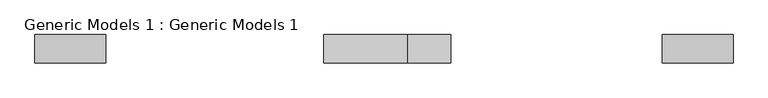
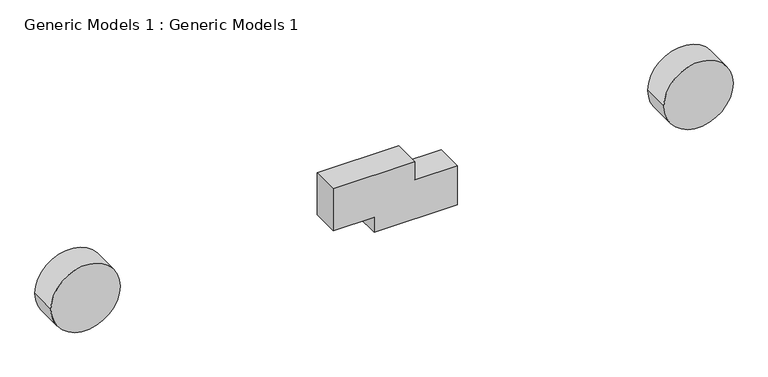
"""IFC4 building model written with IfcOpenShell, lengths in millimetres: proxy geometry, Generic Models 1 : Generic Models 1."""

from ifc_helpers import new_model, si_unit, point, frame, frame_2d, origin, place, context, project, spatial, polyline, circle_curve, trimmed, segment, composite_curve, outline, extrude, source, transform, mapped, element, save


def generic_models_1_generic_models_1_a3dca106(model_context):
    return source(origin(), model_context, "Body", "SweptSolid", [
        extrude(outline(composite_curve([segment(trimmed(circle_curve(frame_2d((10235.9646922, -4682.6474137)), 381.0), [point((10235.9646922, -5063.6474137))], [point((10235.9646922, -4301.6474137))], False, "CARTESIAN"), True, "CONTINUOUS"), segment(trimmed(circle_curve(frame_2d((10235.9646922, -4682.6474137)), 381.0), [point((10235.9646922, -4301.6474137))], [point((10235.9646922, -5063.6474137))], False, "CARTESIAN"), True, "CONTINUOUS")], self_intersect=False)), frame((0.0, -6079.7570853, 0.0), z_axis=(0.0, 1.0, 0.0), x_axis=(0.0, 0.0, 1.0)), (0.0, 0.0, 1.0), 304.8),
        extrude(outline(composite_curve([segment(trimmed(circle_curve(frame_2d((10235.9646922, 2060.9550833)), 381.0), [point((10235.9646922, 1679.9550833))], [point((10235.9646922, 2441.9550833))], False, "CARTESIAN"), True, "CONTINUOUS"), segment(trimmed(circle_curve(frame_2d((10235.9646922, 2060.9550833)), 381.0), [point((10235.9646922, 2441.9550833))], [point((10235.9646922, 1679.9550833))], False, "CARTESIAN"), True, "CONTINUOUS")], self_intersect=False)), frame((0.0, -6079.7570853, 0.0), z_axis=(0.0, 1.0, 0.0), x_axis=(0.0, 0.0, 1.0)), (0.0, 0.0, 1.0), 304.8),
        extrude(outline(polyline([(10550.2946097, -1063.2449167), (10550.2946097, -1959.4202105), (10061.7625083, -1959.4202105), (10061.7625083, -1507.7449167), (9884.7889987, -1507.7449167), (9884.7889987, -593.3449167), (10341.9889987, -593.3449167), (10341.9889987, -1063.2449167), (10550.2946097, -1063.2449167)])), frame((0.0, -6079.7570853, 0.0), z_axis=(0.0, 1.0, 0.0), x_axis=(0.0, 0.0, 1.0)), (0.0, 0.0, 1.0), 304.8),
    ])


if __name__ == "__main__":
    model = new_model("IFC4")
    model_context = context("Model", 3, world=origin())
    ifc_project = project(units=[si_unit("LENGTHUNIT", "METRE", prefix="MILLI")], contexts=[model_context])
    site = spatial("IfcSite", under=ifc_project)
    building = spatial("IfcBuilding", under=site)
    placement = place(None, origin())
    generic_models_1_generic_models_1_shape = generic_models_1_generic_models_1_a3dca106(model_context)
    element("IfcBuildingElementProxy", 1, Name="Generic Models 1 : Generic Models 1", ObjectType="Generic Models 1 : Generic Models 1", at=placement, inside=building, context=model_context, shape_type="MappedRepresentation", body=[
        mapped(generic_models_1_generic_models_1_shape, transform((0.0, 0.0, 0.0), x_axis=(1.0, 0.0, 0.0), y_axis=(0.0, 1.0, 0.0), z_axis=(0.0, 0.0, 1.0))),
    ])
    save(model, "model.ifc")

# Revit data of these elements
# Element 1 (IfcBuildingElementProxy, "Generic Models 1 : Generic Models 1")
#   Materials on its faces: "Parking Stripe"
# Materials
#   "Parking Stripe": class "Paint", colour RGB 250 250 91, transparency 0, Cost = 0
